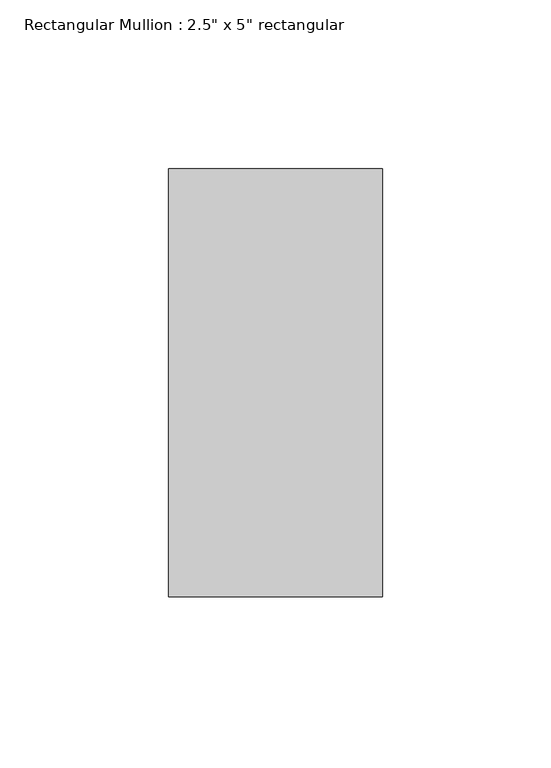
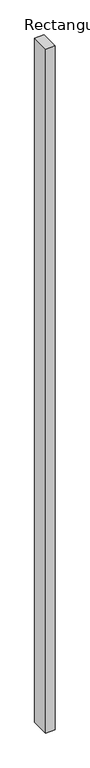
"""IFC4 building model written with IfcOpenShell, lengths in millimetres: member geometry."""

from ifc_helpers import new_model, si_unit, frame, origin, place, context, project, spatial, polyline, outline, extrude, source, transform, mapped, element, save


def member_a0ba9e48(model_context):
    return source(origin(), model_context, "Body", "SweptSolid", [
        extrude(outline(polyline([(0.0, 63.5), (0.0, -63.5), (-63.5, -63.5), (-63.5, 63.5), (0.0, 63.5)])), frame((0.0, 0.0, -4813.3), z_axis=(0.0, 0.0, 1.0), x_axis=(1.0, 0.0, 0.0)), (0.0, 0.0, 1.0), 4813.3),
    ])


if __name__ == "__main__":
    model = new_model("IFC4")
    model_context = context("Model", 3, world=origin())
    ifc_project = project(units=[si_unit("LENGTHUNIT", "METRE", prefix="MILLI")], contexts=[model_context])
    site = spatial("IfcSite", under=ifc_project)
    building = spatial("IfcBuilding", under=site)
    placement = place(None, origin())
    member_shape = member_a0ba9e48(model_context)
    element("IfcMember", 1, ObjectType="Rectangular Mullion : 2.5\" x 5\" rectangular", at=placement, inside=building, context=model_context, shape_type="MappedRepresentation", body=[
        mapped(member_shape, transform((0.0, 0.0, 0.0), x_axis=(1.0, 0.0, 0.0), y_axis=(0.0, 1.0, 0.0), z_axis=(0.0, 0.0, 1.0))),
    ])
    save(model, "model.ifc")

# Revit data of these elements
# Type "Rectangular Mullion : 2.5\" x 5\" rectangular"
#   built-in parameter 1007304 = 0.416667 (stored number, unit not read)
#   built-in parameter 1007301 = 0.104167 (stored number, unit not read)
#   built-in parameter 1007300 = 0.104167 (stored number, unit not read)
# Element 1 (IfcMember, "Rectangular Mullion : 2.5\" x 5\" rectangular")
#   Materials on its faces: "Aluminum"
# Materials
#   "Aluminum": class "Metal", colour RGB 247 247 247, transparency 0, Description = "Aluminum 6061", Cost = 0
